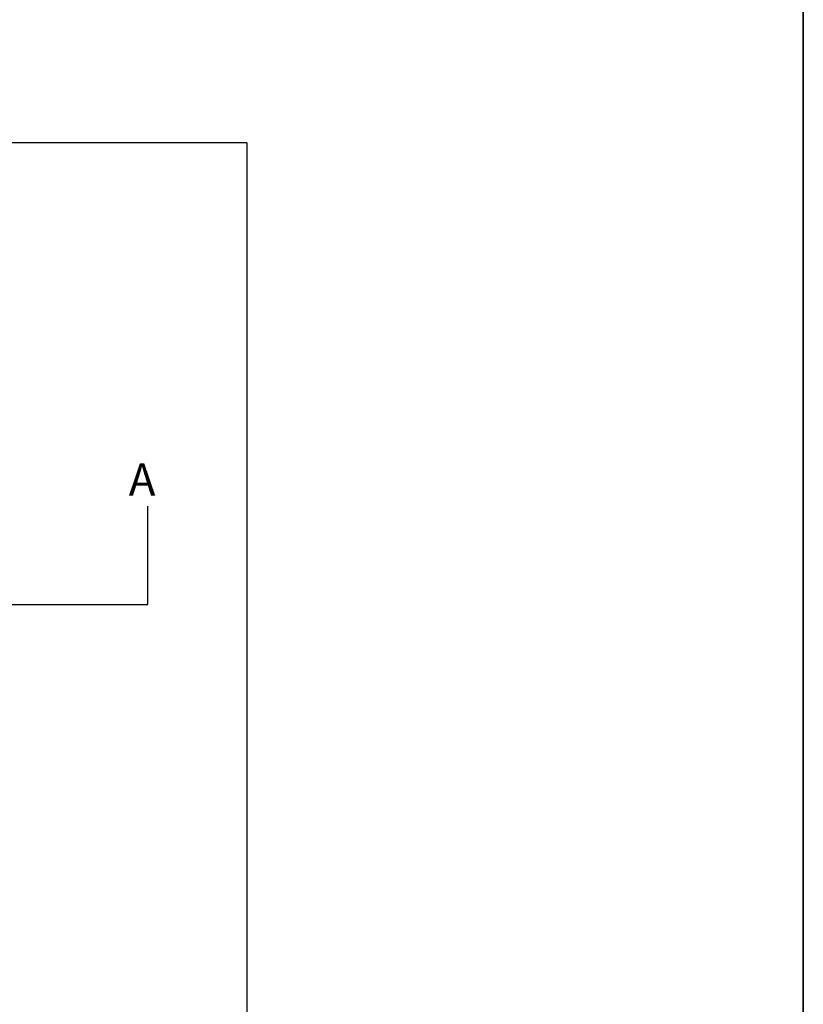
# Model space of a CAD drawing. Units: inches. Extents: x 1944 to 3454, y 1352 to 3055.
# Tile 15 of 17: x 3160 to 3454, y 1900 to 2269. Entities that reach past the tile are written whole.
import ezdxf

# ---------------------------------------------------------------- set-up
doc = ezdxf.new("R2010")
doc.units = ezdxf.units.IN
for name, color, linetype, lineweight in [('A-ANNO-DIMS', 2, 'Continuous', 18), ('A-ANNO-SYMB', 7, 'Continuous', 25), ('A-ANNO-TTLB', 7, 'Continuous', 35)]:
    doc.layers.add(name, color=color, linetype=linetype, lineweight=lineweight)
doc.styles.get("Standard").update_dxf_attribs({"font": 'arial.ttf'})
doc.dimstyles.get("Standard").update_dxf_attribs({"dimtxt": 0.18, "dimasz": 0.18, "dimexe": 0.18, "dimexo": 0.0625, "dimgap": 0.09, "dimtad": 0, "dimtih": 1, "dimtoh": 1, "dimdec": 4, "dimzin": 0, "dimdsep": 46, "dimtxsty": 'Standard', "dimcen": 0.09, "dimadec": 0, "dimazin": 0, "dimtfac": 1, "dimtdec": 4, "dimtofl": 0, "dimtmove": 0, "dimatfit": 3, "dimfxl": 1, "dimtolj": 1, "dimtzin": 0, "dimarcsym": 0})

# ---------------------------------------------------------------- blocks, each defined once
blk = doc.blocks.new('*D187')
at = {"layer": 'A-ANNO-DIMS', "color": 0, "lineweight": -2, "transparency": 16777216}
for p, q in [((3089.53, 2222.6), (3245.46, 2222.6)), ((3245.28, 2222.42), (3245.28, 1856.28)), ((3245.28, 1489.78), (3245.28, 1855.91)), ((3093.18, 1489.6), (3245.46, 1489.6))]:
    blk.add_line(p, q, dxfattribs=at)
at = {"layer": 'A-ANNO-DIMS', "color": 0, "transparency": 16777216}
for points in [[(3245.25, 2222.42), (3245.31, 2222.42), (3245.28, 2222.6)], [(3245.25, 1489.78), (3245.31, 1489.78), (3245.28, 1489.6)]]:
    blk.add_solid(points, dxfattribs=at)
at = {"layer": 'Defpoints', "color": 0, "transparency": 16777216}
for p in [(3089.47, 2222.6), (3245.28, 2222.6), (3093.12, 1489.6)]:
    blk.add_point(p, dxfattribs=at)
at = {"layer": 'A-ANNO-DIMS', "color": 0, "transparency": 16777216, "insert": (3245.28, 1856.1), "char_height": 0.18, "attachment_point": 5}
blk.add_mtext('\\A1;733', dxfattribs=at)

msp = doc.modelspace()

# ---------------------------------------------------------------- linework, layer by layer
at = {"layer": 'A-ANNO-SYMB'}
for p, q in [((3208.282, 2049.778), (3208.282, 2086.587)), ((2622.416, 2049.778), (3208.282, 2049.778))]:
    msp.add_line(p, q, dxfattribs=at)
at = {"layer": 'A-ANNO-TTLB'}
msp.add_lwpolyline([(1943.914, 3054.605), (3453.633, 3054.605), (3453.633, 1351.76), (1943.914, 1351.76)], close=True, dxfattribs=at)

# ---------------------------------------------------------------- texts
at = {"layer": 'A-ANNO-SYMB', "insert": (3201.153, 2102.502), "char_height": 12, "attachment_point": 1}
msp.add_mtext_dynamic_manual_height_columns('A', width=39.53149, gutter_width=12.5, heights=[0], dxfattribs=at)

# ---------------------------------------------------------------- dimensions: what is measured, and where the dimension line sits
at = {"layer": 'A-ANNO-DIMS'}
dim = msp.add_linear_dim(base=(3245.282, 2222.596), p1=(3093.12, 1489.596), p2=(3089.47, 2222.596), angle=90, dimstyle='Standard', override={"dimdec": 0, "dimlfac": 1, "dimrnd": 0, "dimzin": 0, "dimdsep": 46, "dimlunit": 2}, dxfattribs=at)
dim.commit()
dim.dimension.update_dxf_attribs({"geometry": '*D187', "text_midpoint": (3245.282, 1856.096)})

doc.saveas('drawing.dxf')
